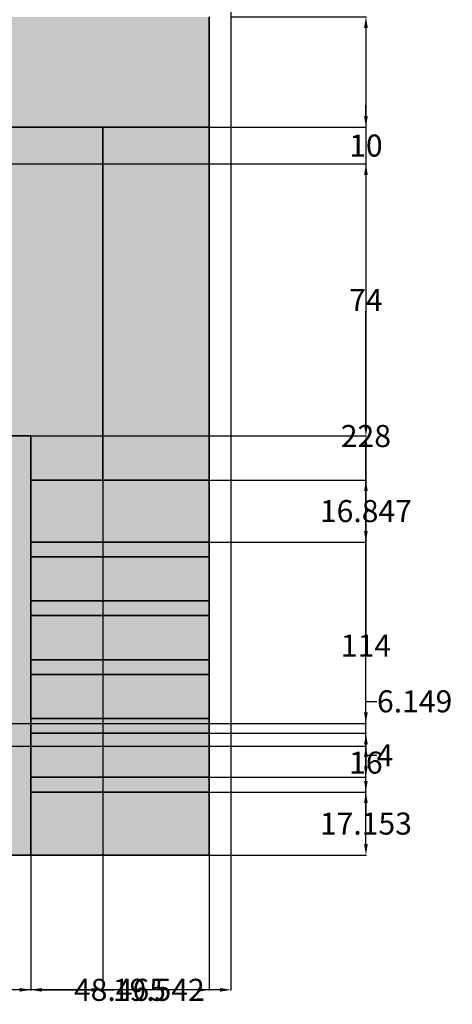
# Model space of a CAD drawing. Units: inches. Extents: x 126 to 726, y 86 to 888.
# Tile 5 of 13: x 609 to 726, y 86 to 354. Entities that reach past the tile are written whole.
import ezdxf

# ---------------------------------------------------------------- set-up
doc = ezdxf.new("R2010")
doc.units = ezdxf.units.IN
doc.header["$MEASUREMENT"] = 0
for name, color, linetype, lineweight in [('A-ANNO-DIMS', 2, 'Continuous', 18), ('A-ELEV', 7, 'Continuous', 35), ('A-ELEV-PATT', 8, 'Continuous', 13)]:
    doc.layers.add(name, color=color, linetype=linetype, lineweight=lineweight)
doc.styles.get("Standard").update_dxf_attribs({"font": 'arial.ttf'})
doc.dimstyles.get("Standard").update_dxf_attribs({"dimtxt": 6, "dimasz": 3, "dimexe": 0.18, "dimexo": 0.0625, "dimgap": 0.09, "dimtad": 0, "dimtih": 1, "dimtoh": 1, "dimdec": 0, "dimzin": 0, "dimdsep": 46, "dimlunit": 3, "dimtxsty": 'Standard', "dimcen": 0.09, "dimadec": 0, "dimazin": 0, "dimtfac": 1, "dimtdec": 0, "dimtofl": 0, "dimtmove": 0, "dimatfit": 3, "dimfxl": 1, "dimtolj": 1, "dimtzin": 0, "dimarcsym": 0})

# ---------------------------------------------------------------- blocks, each defined once
blk = doc.blocks.new('*D13')
at = {"layer": 'A-ANNO-DIMS', "color": 0, "lineweight": -2, "transparency": 16777216}
for p, q in [((665.97, 642.98), (665.97, 90.21)), ((185.97, 126.98), (185.97, 90.21)), ((188.97, 90.39), (419.15, 90.39)), ((662.97, 90.39), (432.8, 90.39))]:
    blk.add_line(p, q, dxfattribs=at)
at = {"layer": 'A-ANNO-DIMS', "color": 0, "transparency": 16777216}
for points in [[(188.97, 90.89), (188.97, 89.89), (185.97, 90.39)], [(662.97, 90.89), (662.97, 89.89), (665.97, 90.39)]]:
    blk.add_solid(points, dxfattribs=at)
at = {"layer": 'Defpoints', "color": 0, "transparency": 16777216}
for p in [(665.97, 643.04), (185.97, 127.04), (665.97, 90.39)]:
    blk.add_point(p, dxfattribs=at)
at = {"layer": 'A-ANNO-DIMS', "color": 0, "transparency": 16777216, "insert": (425.97, 90.39), "char_height": 6, "attachment_point": 5}
blk.add_mtext('\\A1;480', dxfattribs=at)
blk = doc.blocks.new('*D28')
at = {"layer": 'A-ANNO-DIMS', "color": 0, "lineweight": -2, "transparency": 16777216}
for p, q in [((666.04, 355.04), (702.8, 355.04)), ((702.62, 352.04), (702.62, 244.2)), ((702.62, 130.04), (702.62, 237.89)), ((660.11, 127.04), (702.8, 127.04))]:
    blk.add_line(p, q, dxfattribs=at)
at = {"layer": 'A-ANNO-DIMS', "color": 0, "transparency": 16777216}
for points in [[(702.12, 352.04), (703.12, 352.04), (702.62, 355.04)], [(702.12, 130.04), (703.12, 130.04), (702.62, 127.04)]]:
    blk.add_solid(points, dxfattribs=at)
at = {"layer": 'Defpoints', "color": 0, "transparency": 16777216}
for p in [(665.97, 355.04), (702.62, 355.04), (660.05, 127.04)]:
    blk.add_point(p, dxfattribs=at)
at = {"layer": 'A-ANNO-DIMS', "color": 0, "transparency": 16777216, "insert": (702.62, 241.04), "char_height": 6, "attachment_point": 5}
blk.add_mtext('\\A1;228', dxfattribs=at)
blk = doc.blocks.new('*D40')
at = {"layer": 'A-ANNO-DIMS', "color": 0, "lineweight": -2, "transparency": 16777216}
for p, q in [((702.62, 165.86), (702.62, 168.86)), ((702.62, 168.86), (705.62, 168.86)), ((346.12, 162.86), (702.8, 162.86)), ((363.55, 156.71), (702.8, 156.71)), ((702.62, 153.71), (702.62, 150.71))]:
    blk.add_line(p, q, dxfattribs=at)
at = {"layer": 'A-ANNO-DIMS', "color": 0, "transparency": 16777216}
for points in [[(702.12, 165.86), (703.12, 165.86), (702.62, 162.86)], [(702.12, 153.71), (703.12, 153.71), (702.62, 156.71)]]:
    blk.add_solid(points, dxfattribs=at)
at = {"layer": 'Defpoints', "color": 0, "transparency": 16777216}
for p in [(346.06, 162.86), (702.62, 162.86), (363.49, 156.71)]:
    blk.add_point(p, dxfattribs=at)
at = {"layer": 'A-ANNO-DIMS', "color": 0, "transparency": 16777216, "insert": (715.86, 168.86), "char_height": 6, "attachment_point": 5}
blk.add_mtext('\\A1;6.149', dxfattribs=at)
blk = doc.blocks.new('*D42')
at = {"layer": 'A-ANNO-DIMS', "color": 0, "lineweight": -2, "transparency": 16777216}
for p, q in [((429.97, 354.98), (429.97, 90.21)), ((665.97, 354.98), (665.97, 90.21)), ((432.97, 90.39), (541.21, 90.39)), ((662.97, 90.39), (554.74, 90.39))]:
    blk.add_line(p, q, dxfattribs=at)
at = {"layer": 'A-ANNO-DIMS', "color": 0, "transparency": 16777216}
for points in [[(432.97, 90.89), (432.97, 89.89), (429.97, 90.39)], [(662.97, 90.89), (662.97, 89.89), (665.97, 90.39)]]:
    blk.add_solid(points, dxfattribs=at)
at = {"layer": 'Defpoints', "color": 0, "transparency": 16777216}
for p in [(429.97, 355.04), (665.97, 355.04), (665.97, 90.39)]:
    blk.add_point(p, dxfattribs=at)
at = {"layer": 'A-ANNO-DIMS', "color": 0, "transparency": 16777216, "insert": (547.97, 90.39), "char_height": 6, "attachment_point": 5}
blk.add_mtext('\\A1;236', dxfattribs=at)
blk = doc.blocks.new('*D45')
at = {"layer": 'A-ANNO-DIMS', "color": 0, "lineweight": -2, "transparency": 16777216}
for p, q in [((702.624909, 370.042369), (702.624909, 373.042369)), ((666.037409, 367.042369), (702.804909, 367.042369)), ((666.037409, 355.042369), (702.804909, 355.042369)), ((702.624909, 352.042369), (702.624909, 349.042369))]:
    blk.add_line(p, q, dxfattribs=at)
at = {"layer": 'A-ANNO-DIMS', "color": 0, "transparency": 16777216}
for points in [[(702.124909, 370.042369), (703.124909, 370.042369), (702.624909, 367.042369)], [(702.124909, 352.042369), (703.124909, 352.042369), (702.624909, 355.042369)]]:
    blk.add_solid(points, dxfattribs=at)
at = {"layer": 'Defpoints', "color": 0, "transparency": 16777216}
for p in [(665.974909, 367.042369), (702.624909, 367.042369), (665.974909, 355.042369)]:
    blk.add_point(p, dxfattribs=at)
at = {"layer": 'A-ANNO-DIMS', "color": 0, "transparency": 16777216, "insert": (702.624909, 361.042369), "char_height": 6, "attachment_point": 5}
blk.add_mtext('\\A1;12', dxfattribs=at)
blk = doc.blocks.new('*D66')
at = {"layer": 'A-ANNO-DIMS', "color": 0, "lineweight": -2, "transparency": 16777216}
for p, q in [((585.644259, 315.042369), (702.804909, 315.042369)), ((702.624909, 312.042369), (702.624909, 281.132369)), ((702.624909, 244.042369), (702.624909, 274.952369)), ((585.644259, 241.042369), (702.804909, 241.042369))]:
    blk.add_line(p, q, dxfattribs=at)
at = {"layer": 'A-ANNO-DIMS', "color": 0, "transparency": 16777216}
for points in [[(702.124909, 312.042369), (703.124909, 312.042369), (702.624909, 315.042369)], [(702.124909, 244.042369), (703.124909, 244.042369), (702.624909, 241.042369)]]:
    blk.add_solid(points, dxfattribs=at)
at = {"layer": 'Defpoints', "color": 0, "transparency": 16777216}
for p in [(585.581759, 315.042369), (702.624909, 315.042369), (585.581759, 241.042369)]:
    blk.add_point(p, dxfattribs=at)
at = {"layer": 'A-ANNO-DIMS', "color": 0, "transparency": 16777216, "insert": (702.624909, 278.042369), "char_height": 6, "attachment_point": 5}
blk.add_mtext('\\A1;74', dxfattribs=at)
blk = doc.blocks.new('*D67')
at = {"layer": 'A-ANNO-DIMS', "color": 0, "lineweight": -2, "transparency": 16777216}
for p, q in [((702.624909, 328.042369), (702.624909, 331.042369)), ((631.186514, 325.042369), (702.804909, 325.042369)), ((585.644259, 315.042369), (702.804909, 315.042369)), ((702.624909, 312.042369), (702.624909, 309.042369))]:
    blk.add_line(p, q, dxfattribs=at)
at = {"layer": 'A-ANNO-DIMS', "color": 0, "transparency": 16777216}
for points in [[(702.124909, 328.042369), (703.124909, 328.042369), (702.624909, 325.042369)], [(702.124909, 312.042369), (703.124909, 312.042369), (702.624909, 315.042369)]]:
    blk.add_solid(points, dxfattribs=at)
at = {"layer": 'Defpoints', "color": 0, "transparency": 16777216}
for p in [(631.124014, 325.042369), (702.624909, 325.042369), (585.581759, 315.042369)]:
    blk.add_point(p, dxfattribs=at)
at = {"layer": 'A-ANNO-DIMS', "color": 0, "transparency": 16777216, "insert": (702.624909, 320.042369), "char_height": 6, "attachment_point": 5}
blk.add_mtext('\\A1;10', dxfattribs=at)
blk = doc.blocks.new('*D68')
at = {"layer": 'A-ANNO-DIMS', "color": 0, "lineweight": -2, "transparency": 16777216}
for p, q in [((631.12, 324.98), (631.12, 90.21)), ((611.58, 240.98), (611.58, 90.21)), ((614.58, 90.39), (628.12, 90.39)), ((631.12, 90.39), (634.12, 90.39))]:
    blk.add_line(p, q, dxfattribs=at)
at = {"layer": 'A-ANNO-DIMS', "color": 0, "transparency": 16777216}
for points in [[(614.58, 90.89), (614.58, 89.89), (611.58, 90.39)], [(628.12, 90.89), (628.12, 89.89), (631.12, 90.39)]]:
    blk.add_solid(points, dxfattribs=at)
at = {"layer": 'Defpoints', "color": 0, "transparency": 16777216}
for p in [(631.12, 325.04), (611.58, 241.04), (631.12, 90.39)]:
    blk.add_point(p, dxfattribs=at)
at = {"layer": 'A-ANNO-DIMS', "color": 0, "transparency": 16777216, "insert": (646.36, 90.39), "char_height": 6, "attachment_point": 5}
blk.add_mtext('\\A1;19.542', dxfattribs=at)
blk = doc.blocks.new('*D69')
at = {"layer": 'A-ANNO-DIMS', "color": 0, "lineweight": -2, "transparency": 16777216}
for p, q in [((485.97, 126.98), (485.97, 90.21)), ((611.58, 126.98), (611.58, 90.21)), ((488.97, 90.39), (538.85, 90.39)), ((608.58, 90.39), (558.71, 90.39))]:
    blk.add_line(p, q, dxfattribs=at)
at = {"layer": 'A-ANNO-DIMS', "color": 0, "transparency": 16777216}
for points in [[(488.97, 90.89), (488.97, 89.89), (485.97, 90.39)], [(608.58, 90.89), (608.58, 89.89), (611.58, 90.39)]]:
    blk.add_solid(points, dxfattribs=at)
at = {"layer": 'Defpoints', "color": 0, "transparency": 16777216}
for p in [(485.97, 127.04), (611.58, 127.04), (611.58, 90.39)]:
    blk.add_point(p, dxfattribs=at)
at = {"layer": 'A-ANNO-DIMS', "color": 0, "transparency": 16777216, "insert": (548.78, 90.39), "char_height": 6, "attachment_point": 5}
blk.add_mtext('\\A1;125.6', dxfattribs=at)
blk = doc.blocks.new('*D70')
at = {"layer": 'A-ANNO-DIMS', "color": 0, "lineweight": -2, "transparency": 16777216}
for p, q in [((611.64, 241.04), (702.8, 241.04)), ((702.62, 238.04), (702.62, 187.14)), ((702.62, 130.04), (702.62, 180.94)), ((611.64, 127.04), (702.8, 127.04))]:
    blk.add_line(p, q, dxfattribs=at)
at = {"layer": 'A-ANNO-DIMS', "color": 0, "transparency": 16777216}
for points in [[(702.12, 238.04), (703.12, 238.04), (702.62, 241.04)], [(702.12, 130.04), (703.12, 130.04), (702.62, 127.04)]]:
    blk.add_solid(points, dxfattribs=at)
at = {"layer": 'Defpoints', "color": 0, "transparency": 16777216}
for p in [(611.58, 241.04), (702.62, 241.04), (611.58, 127.04)]:
    blk.add_point(p, dxfattribs=at)
at = {"layer": 'A-ANNO-DIMS', "color": 0, "transparency": 16777216, "insert": (702.62, 184.04), "char_height": 6, "attachment_point": 5}
blk.add_mtext('\\A1;114', dxfattribs=at)
blk = doc.blocks.new('*D74')
at = {"layer": 'A-ANNO-DIMS', "color": 0, "lineweight": -2, "transparency": 16777216}
for p, q in [((660.11, 144.2), (702.8, 144.2)), ((702.62, 141.2), (702.62, 138.77)), ((702.62, 130.04), (702.62, 132.46)), ((660.11, 127.04), (702.8, 127.04))]:
    blk.add_line(p, q, dxfattribs=at)
at = {"layer": 'A-ANNO-DIMS', "color": 0, "transparency": 16777216}
for points in [[(702.12, 141.2), (703.12, 141.2), (702.62, 144.2)], [(702.12, 130.04), (703.12, 130.04), (702.62, 127.04)]]:
    blk.add_solid(points, dxfattribs=at)
at = {"layer": 'Defpoints', "color": 0, "transparency": 16777216}
for p in [(660.05, 144.2), (702.62, 144.2), (660.05, 127.04)]:
    blk.add_point(p, dxfattribs=at)
at = {"layer": 'A-ANNO-DIMS', "color": 0, "transparency": 16777216, "insert": (702.62, 135.62), "char_height": 6, "attachment_point": 5}
blk.add_mtext('\\A1;17.153', dxfattribs=at)
blk = doc.blocks.new('*D75')
at = {"layer": 'A-ANNO-DIMS', "color": 0, "lineweight": -2, "transparency": 16777216}
for p, q in [((660.11, 160.2), (702.8, 160.2)), ((702.62, 157.2), (702.62, 155.35)), ((702.62, 147.2), (702.62, 149.04)), ((660.11, 144.2), (702.8, 144.2))]:
    blk.add_line(p, q, dxfattribs=at)
at = {"layer": 'A-ANNO-DIMS', "color": 0, "transparency": 16777216}
for points in [[(702.12, 157.2), (703.12, 157.2), (702.62, 160.2)], [(702.12, 147.2), (703.12, 147.2), (702.62, 144.2)]]:
    blk.add_solid(points, dxfattribs=at)
at = {"layer": 'Defpoints', "color": 0, "transparency": 16777216}
for p in [(660.05, 160.2), (702.62, 160.2), (660.05, 144.2)]:
    blk.add_point(p, dxfattribs=at)
at = {"layer": 'A-ANNO-DIMS', "color": 0, "transparency": 16777216, "insert": (702.62, 152.2), "char_height": 6, "attachment_point": 5}
blk.add_mtext('\\A1;16', dxfattribs=at)
blk = doc.blocks.new('*D76')
at = {"layer": 'A-ANNO-DIMS', "color": 0, "lineweight": -2, "transparency": 16777216}
for p, q in [((660.11, 229.04), (702.8, 229.04)), ((702.62, 226.04), (702.62, 223.77)), ((702.62, 215.2), (702.62, 217.47)), ((660.11, 212.2), (702.8, 212.2))]:
    blk.add_line(p, q, dxfattribs=at)
at = {"layer": 'A-ANNO-DIMS', "color": 0, "transparency": 16777216}
for points in [[(702.12, 226.04), (703.12, 226.04), (702.62, 229.04)], [(702.12, 215.2), (703.12, 215.2), (702.62, 212.2)]]:
    blk.add_solid(points, dxfattribs=at)
at = {"layer": 'Defpoints', "color": 0, "transparency": 16777216}
for p in [(660.05, 229.04), (702.62, 229.04), (660.05, 212.2)]:
    blk.add_point(p, dxfattribs=at)
at = {"layer": 'A-ANNO-DIMS', "color": 0, "transparency": 16777216, "insert": (702.62, 220.62), "char_height": 6, "attachment_point": 5}
blk.add_mtext('\\A1;16.847', dxfattribs=at)
blk = doc.blocks.new('*D77')
at = {"layer": 'A-ANNO-DIMS', "color": 0, "lineweight": -2, "transparency": 16777216}
for p, q in [((702.62, 151.2), (702.62, 154.2)), ((702.62, 154.2), (705.62, 154.2)), ((611.64, 148.2), (702.8, 148.2)), ((611.64, 144.2), (702.8, 144.2)), ((702.62, 141.2), (702.62, 138.2))]:
    blk.add_line(p, q, dxfattribs=at)
at = {"layer": 'A-ANNO-DIMS', "color": 0, "transparency": 16777216}
for points in [[(702.12, 151.2), (703.12, 151.2), (702.62, 148.2)], [(702.12, 141.2), (703.12, 141.2), (702.62, 144.2)]]:
    blk.add_solid(points, dxfattribs=at)
at = {"layer": 'Defpoints', "color": 0, "transparency": 16777216}
for p in [(611.58, 148.2), (702.62, 148.2), (611.58, 144.2)]:
    blk.add_point(p, dxfattribs=at)
at = {"layer": 'A-ANNO-DIMS', "color": 0, "transparency": 16777216, "insert": (707.79, 154.2), "char_height": 6, "attachment_point": 5}
blk.add_mtext('\\A1;4', dxfattribs=at)
blk = doc.blocks.new('*D78')
at = {"layer": 'A-ANNO-DIMS', "color": 0, "lineweight": -2, "transparency": 16777216}
for p, q in [((611.58, 228.98), (611.58, 90.21)), ((660.05, 228.98), (660.05, 90.21)), ((614.58, 90.39), (623.13, 90.39)), ((657.05, 90.39), (648.5, 90.39))]:
    blk.add_line(p, q, dxfattribs=at)
at = {"layer": 'A-ANNO-DIMS', "color": 0, "transparency": 16777216}
for points in [[(614.58, 90.89), (614.58, 89.89), (611.58, 90.39)], [(657.05, 90.89), (657.05, 89.89), (660.05, 90.39)]]:
    blk.add_solid(points, dxfattribs=at)
at = {"layer": 'Defpoints', "color": 0, "transparency": 16777216}
for p in [(611.58, 229.04), (660.05, 229.04), (660.05, 90.39)]:
    blk.add_point(p, dxfattribs=at)
at = {"layer": 'A-ANNO-DIMS', "color": 0, "transparency": 16777216, "insert": (635.81, 90.39), "char_height": 6, "attachment_point": 5}
blk.add_mtext('\\A1;48.465', dxfattribs=at)

msp = doc.modelspace()

# ---------------------------------------------------------------- hatches: boundary and pattern name
at = {"layer": 'A-ELEV-PATT'}
h = msp.add_hatch(color=256, dxfattribs=at)
h.dxf.hatch_style = 1
h.paths.add_polyline_path([(485.9749, 595.0424), (485.9749, 564.6845), (585.5818, 564.6845), (585.5818, 595.0424)])
h.paths.add_polyline_path([(660.0469, 325.0424), (660.0469, 355.0424), (485.9749, 355.0424), (485.9749, 325.0424)])
h = msp.add_hatch(color=256, dxfattribs=at)
h.dxf.hatch_style = 1
h.paths.add_polyline_path([(631.124, 325.0424), (485.9749, 325.0424), (485.9749, 315.0424), (585.5818, 315.0424), (585.5818, 241.0424), (611.5818, 241.0424), (611.5818, 229.0424), (631.124, 229.0424)])
h = msp.add_hatch(color=256, dxfattribs=at)
h.dxf.hatch_style = 1
h.paths.add_polyline_path([(631.124, 325.0424), (585.5818, 325.0424), (585.5818, 241.0424), (611.5818, 241.0424), (611.5818, 229.0424), (631.124, 229.0424)])
h = msp.add_hatch(color=256, dxfattribs=at)
h.dxf.hatch_style = 1
h.paths.add_polyline_path([(660.0469, 325.0424), (631.124, 325.0424), (631.124, 229.0424), (660.0469, 229.0424)])
h.paths.add_polyline_path([(660.0469, 212.1951), (611.5818, 212.1951), (611.5818, 208.1951), (660.0469, 208.1951)])
h.paths.add_polyline_path([(660.0469, 196.1951), (611.5818, 196.1951), (611.5818, 192.1951), (660.0469, 192.1951)])
h.paths.add_polyline_path([(660.0469, 180.1951), (611.5818, 180.1951), (611.5818, 176.1951), (660.0469, 176.1951)])
h.paths.add_polyline_path([(660.0469, 164.1951), (611.5818, 164.1951), (611.5818, 160.1951), (660.0469, 160.1951)])
h.paths.add_polyline_path([(660.0469, 148.1951), (611.5818, 148.1951), (611.5818, 144.1951), (660.0469, 144.1951)])
h = msp.add_hatch(color=256, dxfattribs=at)
h.dxf.hatch_style = 1
h.paths.add_polyline_path([(611.5818, 241.0424), (485.9749, 241.0424), (485.9749, 127.0424), (611.5818, 127.0424), (611.5818, 229.0424)])
h.paths.add_polyline_path([(505.9749, 235.0424), (513.9749, 235.0424), (513.9749, 133.0424), (505.9749, 133.0424)], flags=16)
h.paths.add_polyline_path([(499.9749, 235.0424), (499.9749, 133.0424), (491.9749, 133.0424), (491.9749, 235.0424)], flags=16)
h.paths.add_polyline_path([(519.9749, 235.0424), (527.9749, 235.0424), (527.9749, 133.0424), (519.9749, 133.0424)], flags=16)
h.paths.add_polyline_path([(533.9749, 235.0424), (605.5818, 235.0424), (605.5818, 133.0424), (533.9749, 133.0424)], flags=16)
h = msp.add_hatch(color=256, dxfattribs=at)
h.dxf.hatch_style = 1
h.paths.add_polyline_path([(660.0469, 144.1951), (611.5818, 144.1951), (611.5818, 127.0424), (660.0469, 127.0424)])
h.paths.add_polyline_path([(660.0469, 160.1951), (611.5818, 160.1951), (611.5818, 148.1951), (660.0469, 148.1951)])
h.paths.add_polyline_path([(660.0469, 176.1951), (611.5818, 176.1951), (611.5818, 164.1951), (660.0469, 164.1951)])
h.paths.add_polyline_path([(660.0469, 192.1951), (611.5818, 192.1951), (611.5818, 180.1951), (660.0469, 180.1951)])
h.paths.add_polyline_path([(660.0469, 208.1951), (611.5818, 208.1951), (611.5818, 196.1951), (660.0469, 196.1951)])
h.paths.add_polyline_path([(660.0469, 229.0424), (611.5818, 229.0424), (611.5818, 212.1951), (660.0469, 212.1951)])

# ---------------------------------------------------------------- linework, layer by layer
at = {"layer": 'A-ELEV'}
for p, q in [((660.0469, 355.0424), (660.0469, 127.0424)), ((660.0469, 325.0424), (485.9749, 325.0424)), ((631.124, 229.0424), (631.124, 325.0424)), ((611.5818, 241.0424), (485.9749, 241.0424)), ((611.5818, 229.0424), (611.5818, 241.0424)), ((660.0469, 229.0424), (611.5818, 229.0424)), ((611.5818, 229.0424), (611.5818, 127.0424)), ((660.0469, 212.1951), (611.5818, 212.1951)), ((660.0469, 208.1951), (611.5818, 208.1951)), ((660.0469, 196.1951), (611.5818, 196.1951)), ((660.0469, 192.1951), (611.5818, 192.1951)), ((660.0469, 180.1951), (611.5818, 180.1951)), ((660.0469, 176.1951), (611.5818, 176.1951)), ((660.0469, 164.1951), (611.5818, 164.1951)), ((660.0469, 160.1951), (611.5818, 160.1951)), ((660.0469, 148.1951), (611.5818, 148.1951)), ((660.0469, 144.1951), (611.5818, 144.1951)), ((185.9749, 127.0424), (660.0469, 127.0424))]:
    msp.add_line(p, q, dxfattribs=at)

# ---------------------------------------------------------------- dimensions: what is measured, and where the dimension line sits
at = {"layer": 'A-ANNO-DIMS'}
for base, p1, p2, override, picture, middle in [((665.9749, 90.3924), (185.9749, 127.0424), (665.9749, 643.0424), {"dimdec": 0, "dimlfac": 1, "dimrnd": 0, "dimzin": 0, "dimdsep": 46, "dimlunit": 2}, '*D13', (425.9749, 90.3924)), ((665.9749, 90.3924), (429.9749, 355.0424), (665.9749, 355.0424), {"dimdec": 0, "dimlfac": 1, "dimrnd": 0, "dimzin": 0, "dimdsep": 46, "dimlunit": 2}, '*D42', (547.9749, 90.3924)), ((631.124, 90.3924), (611.5818, 241.0424), (631.124, 325.0424), {"dimdec": 3, "dimlfac": 1, "dimrnd": 0, "dimzin": 0, "dimdsep": 46, "dimlunit": 2}, '*D68', (646.3552, 90.3924)), ((660.0469, 90.3924), (611.5818, 229.0424), (660.0469, 229.0424), {"dimdec": 3, "dimlfac": 1, "dimrnd": 0, "dimzin": 0, "dimdsep": 46, "dimlunit": 2}, '*D78', (635.8143, 90.3924)), ((611.5818, 90.3924), (485.9749, 127.0424), (611.5818, 127.0424), {"dimdec": 1, "dimlfac": 1, "dimrnd": 0, "dimzin": 0, "dimdsep": 46, "dimlunit": 2}, '*D69', (548.7783, 90.3924))]:
    dim = msp.add_linear_dim(base=base, p1=p1, p2=p2, dimstyle='Standard', override=override, dxfattribs=at)
    dim.commit()
    dim.dimension.update_dxf_attribs({"geometry": picture, "text_midpoint": middle})
for base, p1, p2, override, picture, middle in [((702.6249, 367.0424), (665.9749, 355.0424), (665.9749, 367.0424), {"dimdec": 0, "dimlfac": 1, "dimrnd": 0, "dimzin": 0, "dimdsep": 46, "dimlunit": 2}, '*D45', (702.6249, 361.0424)), ((702.6249, 355.0424), (660.0469, 127.0424), (665.9749, 355.0424), {"dimdec": 0, "dimlfac": 1, "dimrnd": 0, "dimzin": 0, "dimdsep": 46, "dimlunit": 2}, '*D28', (702.6249, 241.0424)), ((702.6249, 325.0424), (585.5818, 315.0424), (631.124, 325.0424), {"dimdec": 0, "dimlfac": 1, "dimrnd": 0, "dimzin": 0, "dimdsep": 46, "dimlunit": 2}, '*D67', (702.6249, 320.0424)), ((702.6249, 315.0424), (585.5818, 241.0424), (585.5818, 315.0424), {"dimdec": 0, "dimlfac": 1, "dimrnd": 0, "dimzin": 0, "dimdsep": 46, "dimlunit": 2}, '*D66', (702.6249, 278.0424)), ((702.6249, 241.0424), (611.5818, 127.0424), (611.5818, 241.0424), {"dimdec": 0, "dimlfac": 1, "dimrnd": 0, "dimzin": 0, "dimdsep": 46, "dimlunit": 2}, '*D70', (702.6249, 184.0424)), ((702.6249, 229.0424), (660.0469, 212.1951), (660.0469, 229.0424), {"dimdec": 3, "dimlfac": 1, "dimrnd": 0, "dimzin": 0, "dimdsep": 46, "dimlunit": 2}, '*D76', (702.6249, 220.6187)), ((702.6249, 162.8622), (363.489, 156.7133), (346.055, 162.8622), {"dimdec": 3, "dimlfac": 1, "dimrnd": 0, "dimzin": 0, "dimdsep": 46, "dimlunit": 2}, '*D40', (715.8609, 168.8622)), ((702.6249, 148.1951), (611.5818, 144.1951), (611.5818, 148.1951), {"dimdec": 0, "dimlfac": 1, "dimrnd": 0, "dimzin": 0, "dimdsep": 46, "dimlunit": 2}, '*D77', (707.7899, 154.1951)), ((702.6249, 160.1951), (660.0469, 144.1951), (660.0469, 160.1951), {"dimdec": 0, "dimlfac": 1, "dimrnd": 0, "dimzin": 0, "dimdsep": 46, "dimlunit": 2}, '*D75', (702.6249, 152.1951)), ((702.6249, 144.1951), (660.0469, 127.0424), (660.0469, 144.1951), {"dimdec": 3, "dimlfac": 1, "dimrnd": 0, "dimzin": 0, "dimdsep": 46, "dimlunit": 2}, '*D74', (702.6249, 135.6187))]:
    dim = msp.add_linear_dim(base=base, p1=p1, p2=p2, angle=90, dimstyle='Standard', override=override, dxfattribs=at)
    dim.commit()
    dim.dimension.update_dxf_attribs({"geometry": picture, "text_midpoint": middle})

doc.saveas('drawing.dxf')
